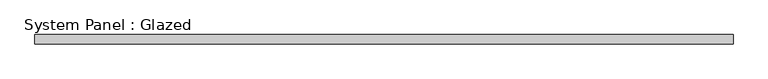
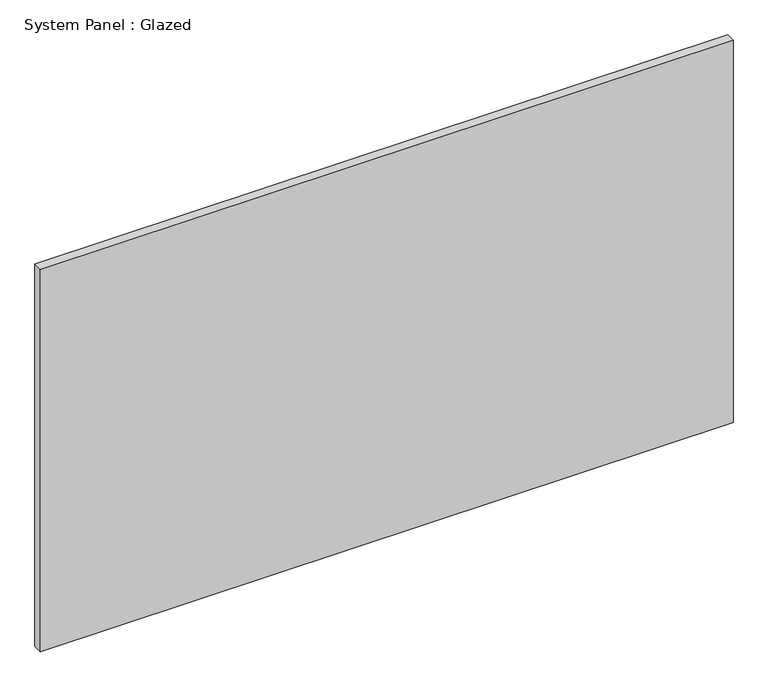
"""IFC4 building model written with IfcOpenShell, lengths in millimetres: plate geometry, System Panel : Glazed."""

from ifc_helpers import new_model, si_unit, origin, origin_with_axes, place, context, project, spatial, polyline, outline, extrude, source, transform, mapped, element, save


def system_panel_glazed_30ab8f14(model_context):
    return source(origin(), model_context, "Body", "SweptSolid", [
        extrude(outline(polyline([(913.5002329, 24.5), (-913.5002329, 24.5), (-913.5002329, 49.5), (913.5002329, 49.5), (913.5002329, 24.5)])), origin_with_axes(), (0.0, 0.0, 1.0), 1066.8),
    ])


if __name__ == "__main__":
    model = new_model("IFC4")
    model_context = context("Model", 3, world=origin())
    ifc_project = project(units=[si_unit("LENGTHUNIT", "METRE", prefix="MILLI")], contexts=[model_context])
    site = spatial("IfcSite", under=ifc_project)
    building = spatial("IfcBuilding", under=site)
    placement = place(None, origin())
    system_panel_glazed_shape = system_panel_glazed_30ab8f14(model_context)
    element("IfcPlate", 1, ObjectType="System Panel : Glazed", at=placement, inside=building, context=model_context, shape_type="MappedRepresentation", body=[
        mapped(system_panel_glazed_shape, transform((0.0, 0.0, 0.0), x_axis=(1.0, 0.0, 0.0), y_axis=(0.0, 1.0, 0.0), z_axis=(0.0, 0.0, 1.0))),
    ])
    save(model, "model.ifc")

# Revit data of these elements
# Type "System Panel : Glazed"
#   Keynote = "H11"
#   Construction Type Id = "GSP4R"
#   Analytic Construction = "1/8 in Pilkington single glazing"
#   Visual Light Transmittance = 0.9
#   Solar Heat Gain Coefficient = 0.86
#   Heat Transfer Coefficient (U) = 6.7069 W/(m²·K)
#   Define Thermal Properties by = 1
# Element 1 (IfcPlate, "System Panel : Glazed")
#   Materials on its faces: "Glass"
# Materials
#   "Glass": class "Glass", colour RGB 0 128 192, transparency 0.9, Description = "Soda Lime Glass", Cost = 0
